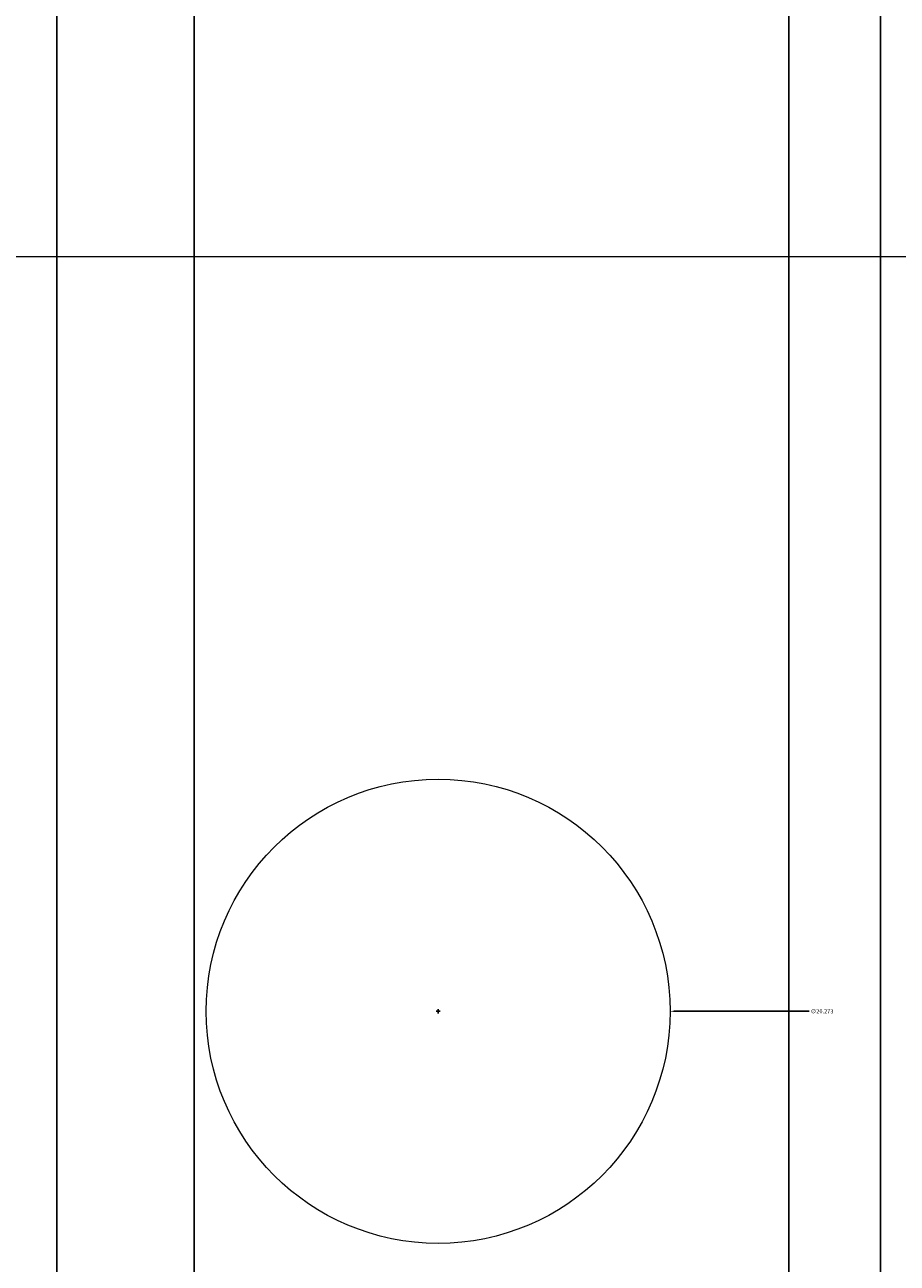
# Model space of a CAD drawing. Units: inches. Extents: x 2231 to 2461, y 2045 to 2455.
# Tile 47 of 95: x 2297 to 2336, y 2217 to 2271. Entities that reach past the tile are written whole.
import ezdxf

# ---------------------------------------------------------------- set-up
doc = ezdxf.new("R2010")
doc.units = ezdxf.units.IN
doc.layers.add('A-ANNO-DIMS', color=2, linetype='Continuous', lineweight=18)
doc.layers.add('A-FURN', color=9, linetype='Continuous', lineweight=18)
doc.styles.get("Standard").update_dxf_attribs({"font": 'arial.ttf'})
doc.dimstyles.get("Standard").update_dxf_attribs({"dimtxt": 0.18, "dimasz": 0.18, "dimexe": 0.18, "dimexo": 0.0625, "dimgap": 0.09, "dimtad": 0, "dimtih": 1, "dimtoh": 1, "dimdec": 4, "dimzin": 0, "dimdsep": 46, "dimtxsty": 'Standard', "dimcen": 0.09, "dimadec": 0, "dimazin": 0, "dimtfac": 1, "dimtdec": 4, "dimtofl": 0, "dimtmove": 0, "dimatfit": 3, "dimfxl": 1, "dimtolj": 1, "dimtzin": 0, "dimarcsym": 0})

# ---------------------------------------------------------------- blocks, each defined once
blk = doc.blocks.new('*D49')
at = {"layer": 'A-ANNO-DIMS', "color": 0, "lineweight": -2, "transparency": 16777216}
for p, q in [((2298.794, 2182.895), (2298.794, 2454.645)), ((2298.974, 2454.465), (2301.644, 2454.465)), ((2304.614, 2454.465), (2301.943, 2454.465)), ((2304.794, 2182.895), (2304.794, 2454.645))]:
    blk.add_line(p, q, dxfattribs=at)
at = {"layer": 'A-ANNO-DIMS', "color": 0, "transparency": 16777216}
for points in [[(2298.974, 2454.495), (2298.974, 2454.435), (2298.794, 2454.465)], [(2304.614, 2454.495), (2304.614, 2454.435), (2304.794, 2454.465)]]:
    blk.add_solid(points, dxfattribs=at)
at = {"layer": 'Defpoints', "color": 0, "transparency": 16777216}
for p in [(2304.794, 2454.465), (2298.794, 2182.833), (2304.794, 2182.833)]:
    blk.add_point(p, dxfattribs=at)
at = {"layer": 'A-ANNO-DIMS', "color": 0, "transparency": 16777216, "insert": (2301.794, 2454.465), "char_height": 0.18, "attachment_point": 5}
blk.add_mtext('\\A1;6', dxfattribs=at)
blk = doc.blocks.new('*D50')
at = {"layer": 'A-ANNO-DIMS', "color": 0, "lineweight": -2, "transparency": 16777216}
for p, q in [((2304.794, 2182.895), (2304.794, 2454.645)), ((2304.974, 2454.465), (2319.575, 2454.465)), ((2334.614, 2454.465), (2320.012, 2454.465)), ((2334.794, 2182.895), (2334.794, 2454.645))]:
    blk.add_line(p, q, dxfattribs=at)
at = {"layer": 'A-ANNO-DIMS', "color": 0, "transparency": 16777216}
for points in [[(2304.974, 2454.495), (2304.974, 2454.435), (2304.794, 2454.465)], [(2334.614, 2454.495), (2334.614, 2454.435), (2334.794, 2454.465)]]:
    blk.add_solid(points, dxfattribs=at)
at = {"layer": 'Defpoints', "color": 0, "transparency": 16777216}
for p in [(2334.794, 2454.465), (2304.794, 2182.833), (2334.794, 2182.833)]:
    blk.add_point(p, dxfattribs=at)
at = {"layer": 'A-ANNO-DIMS', "color": 0, "transparency": 16777216, "insert": (2319.794, 2454.465), "char_height": 0.18, "attachment_point": 5}
blk.add_mtext('\\A1;30', dxfattribs=at)
blk = doc.blocks.new('*D51')
at = {"layer": 'A-ANNO-DIMS', "color": 0, "lineweight": -2, "transparency": 16777216}
for p, q in [((2258.794, 2306.77), (2258.794, 2044.803)), ((2330.794, 2306.77), (2330.794, 2044.803)), ((2258.974, 2044.983), (2294.576, 2044.983)), ((2330.614, 2044.983), (2295.011, 2044.983))]:
    blk.add_line(p, q, dxfattribs=at)
at = {"layer": 'A-ANNO-DIMS', "color": 0, "transparency": 16777216}
for points in [[(2258.974, 2045.013), (2258.974, 2044.953), (2258.794, 2044.983)], [(2330.614, 2045.013), (2330.614, 2044.953), (2330.794, 2044.983)]]:
    blk.add_solid(points, dxfattribs=at)
at = {"layer": 'Defpoints', "color": 0, "transparency": 16777216}
for p in [(2258.794, 2306.833), (2330.794, 2306.833), (2330.794, 2044.983)]:
    blk.add_point(p, dxfattribs=at)
at = {"layer": 'A-ANNO-DIMS', "color": 0, "transparency": 16777216, "insert": (2294.794, 2044.983), "char_height": 0.18, "attachment_point": 5}
blk.add_mtext('\\A1;72', dxfattribs=at)
blk = doc.blocks.new('*D52')
at = {"layer": 'A-ANNO-DIMS', "color": 0, "lineweight": -2, "transparency": 16777216}
for p, q in [((2330.794, 2306.77), (2330.794, 2044.803)), ((2360.794, 2306.77), (2360.794, 2044.803)), ((2330.974, 2044.983), (2345.575, 2044.983)), ((2360.614, 2044.983), (2346.012, 2044.983))]:
    blk.add_line(p, q, dxfattribs=at)
at = {"layer": 'A-ANNO-DIMS', "color": 0, "transparency": 16777216}
for points in [[(2330.974, 2045.013), (2330.974, 2044.953), (2330.794, 2044.983)], [(2360.614, 2045.013), (2360.614, 2044.953), (2360.794, 2044.983)]]:
    blk.add_solid(points, dxfattribs=at)
at = {"layer": 'Defpoints', "color": 0, "transparency": 16777216}
for p in [(2330.794, 2306.833), (2360.794, 2306.833), (2360.794, 2044.983)]:
    blk.add_point(p, dxfattribs=at)
at = {"layer": 'A-ANNO-DIMS', "color": 0, "transparency": 16777216, "insert": (2345.794, 2044.983), "char_height": 0.18, "attachment_point": 5}
blk.add_mtext('\\A1;30', dxfattribs=at)
blk = doc.blocks.new('*D77')
at = {"layer": 'A-ANNO-DIMS', "color": 0, "lineweight": -2, "transparency": 16777216}
for p, q in [((2315.372, 2228.397), (2315.552, 2228.397)), ((2315.462, 2228.307), (2315.462, 2228.487)), ((2331.68, 2228.397), (2325.778, 2228.397))]:
    blk.add_line(p, q, dxfattribs=at)
at = {"layer": 'A-ANNO-DIMS', "color": 0, "transparency": 16777216}
blk.add_solid([(2325.778, 2228.427), (2325.778, 2228.367), (2325.598, 2228.397)], dxfattribs=at)
at = {"layer": 'Defpoints', "color": 0, "transparency": 16777216}
for p in [(2305.325, 2228.398), (2325.598, 2228.397)]:
    blk.add_point(p, dxfattribs=at)
at = {"layer": 'A-ANNO-DIMS', "color": 0, "transparency": 16777216, "insert": (2332.241, 2228.397), "char_height": 0.18, "attachment_point": 5}
blk.add_mtext('\\A1;∅20.273', dxfattribs=at)

msp = doc.modelspace()

# ---------------------------------------------------------------- linework, layer by layer
at = {"layer": 'A-FURN'}
msp.add_lwpolyline([(2285.6353, 2255.1137), (2285.6353, 2261.3584), (2340.6673, 2261.3584), (2340.6673, 2189.3477), (2285.6353, 2189.3477), (2285.6353, 2195.1137)], dxfattribs=at)
msp.add_circle((2315.4615, 2228.3973), 10.1364, dxfattribs=at)

# ---------------------------------------------------------------- dimensions: what is measured, and where the dimension line sits
at = {"layer": 'A-ANNO-DIMS'}
for base, p1, p2, picture, middle in [((2304.7935, 2454.4653), (2298.7935, 2182.8328), (2304.7935, 2182.8328), '*D49', (2301.7935, 2454.4653)), ((2334.7935, 2454.4653), (2304.7935, 2182.8328), (2334.7935, 2182.8328), '*D50', (2319.7935, 2454.4653)), ((2330.7935, 2044.9825), (2258.7935, 2306.8328), (2330.7935, 2306.8328), '*D51', (2294.7935, 2044.9825)), ((2360.7935, 2044.9825), (2330.7935, 2306.8328), (2360.7935, 2306.8328), '*D52', (2345.7935, 2044.9825))]:
    dim = msp.add_linear_dim(base=base, p1=p1, p2=p2, dimstyle='Standard', override={"dimdec": 0, "dimlfac": 1, "dimrnd": 0, "dimzin": 0, "dimdsep": 46, "dimlunit": 2}, dxfattribs=at)
    dim.commit()
    dim.dimension.update_dxf_attribs({"geometry": picture, "text_midpoint": middle})
dim = msp.add_diameter_dim_2p(p1=(2305.3251, 2228.3977), p2=(2325.5979, 2228.397), dimstyle='Standard', override={"dimdec": 3, "dimlfac": 1, "dimrnd": 0, "dimzin": 0, "dimdsep": 46, "dimlunit": 2}, dxfattribs=at)
dim.commit()
dim.dimension.update_dxf_attribs({"geometry": '*D77', "text_midpoint": (2331.6797, 2228.3968), "dimtype": 163})

doc.saveas('drawing.dxf')
